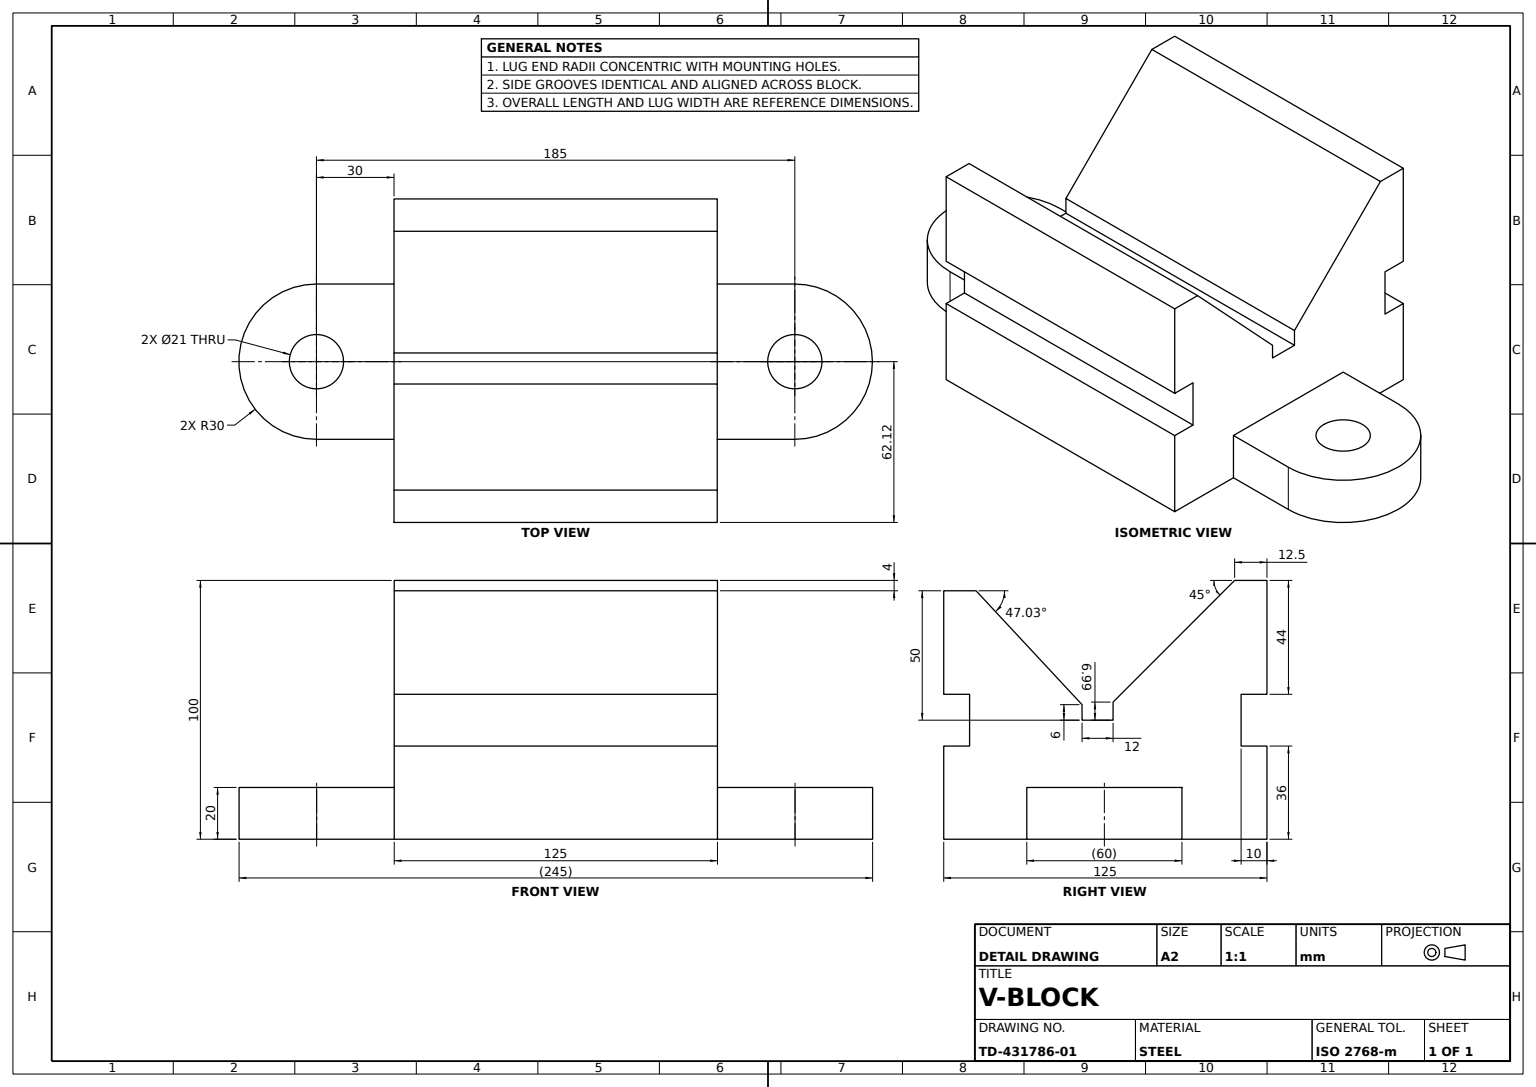
SolidWorks part; units mm, degrees
material "Plain Carbon Steel"
ref_plane "Front Plane" through (0, 0, 0) normal (0, 0, 1) x (1, 0, 0)
ref_plane "Top Plane" through (0, 0, 0) normal (0, 1, 0) x (1, 0, 0)
ref_plane "Right Plane" through (0, 0, 0) normal (1, 0, 0) x (0, 0, -1)
sketch "V-Block Profile Sketch" plane through (0, 0, 0) normal (0, 0, 1) x (1, 0, 0)
  line L0 (-40.458, 0) -> (84.542, 0)
  line L1 (84.542, 0) -> (84.542, 36)
  line L2 (84.542, 36) -> (74.542, 36)
  line L3 (74.542, 36) -> (74.542, 56)
  line L4 (74.542, 56) -> (84.542, 56)
  line L5 (84.542, 56) -> (84.542, 96)
  line L6 (84.542, 96) -> (72.042, 96)
  line L7 (72.042, 96) -> (31.0525, 52)
  line L8 (31.0525, 52) -> (31.0525, 46)
  line L9 (31.0525, 46) -> (19.0525, 46)
  line L10 (19.0525, 46) -> (19.0525, 52.9895)
  line L11 (19.0525, 52.9895) -> (-27.958, 100)
  line L12 (-27.958, 100) -> (-40.458, 100)
  line L13 (-40.458, 100) -> (-40.458, 56)
  line L14 (-40.458, 56) -> (-30.458, 56)
  line L15 (-30.458, 56) -> (-30.458, 36)
  line L16 (-30.458, 36) -> (-40.458, 36)
  line L17 (-40.458, 36) -> (-40.458, 0)
  point P13 (74.542, 46)
  dimension "D1" = 125
  dimension "D2" = 100
  dimension "D3" = 12.5
  dimension "D4" = 44
  dimension "D5" = 50
  dimension "D6" = 6
  dimension "D7" = 12
  dimension "D8" = 20
  dimension "D9" = 20
  dimension "D10" = 36
  dimension "D11" = 36
  dimension "D12" = 10
  dimension "D13" = 10
  dimension "D14" = 10
  dimension "D15" = 50
  dimension "D16" = 45
  dimension "D17" = 6.9895
  dimension "D18" = 40.458
extrude "V-Block Body" add sketch "V-Block Profile Sketch" along normal blind 125
sketch "Mounting Lugs Sketch" plane through (0, 0, 0) normal (0, -1, 0) x (1, 0, 0)
  line L0 (22.4214, 155) -> (22.4214, -30) construction
  line L1 (52.4214, 155) -> (52.4214, -30)
  line L2 (-7.5786, 155) -> (-7.5786, -30)
  line L3 (-40.458, 125) -> (84.542, 125) construction
  line L4 (84.542, 125) -> (84.542, 0) construction
  arc A0 (52.4214, 155) -> (-7.5786, 155) centre (22.4214, 155) ccw
  arc A1 (-7.5786, -30) -> (52.4214, -30) centre (22.4214, -30) ccw
  circle A2 centre (22.4214, 155) radius 10.5
  circle A3 centre (22.4214, -30) radius 10.5
  point P2 (22.4214, 62.5)
  dimension "D4" = 21
  dimension "D5" = 21
  dimension "D1" = 60
  dimension "D2" = 185
  dimension "D3" = 30
  dimension "D6" = 62.1206
extrude "Mounting Lugs" add sketch "Mounting Lugs Sketch" against normal blind 20
